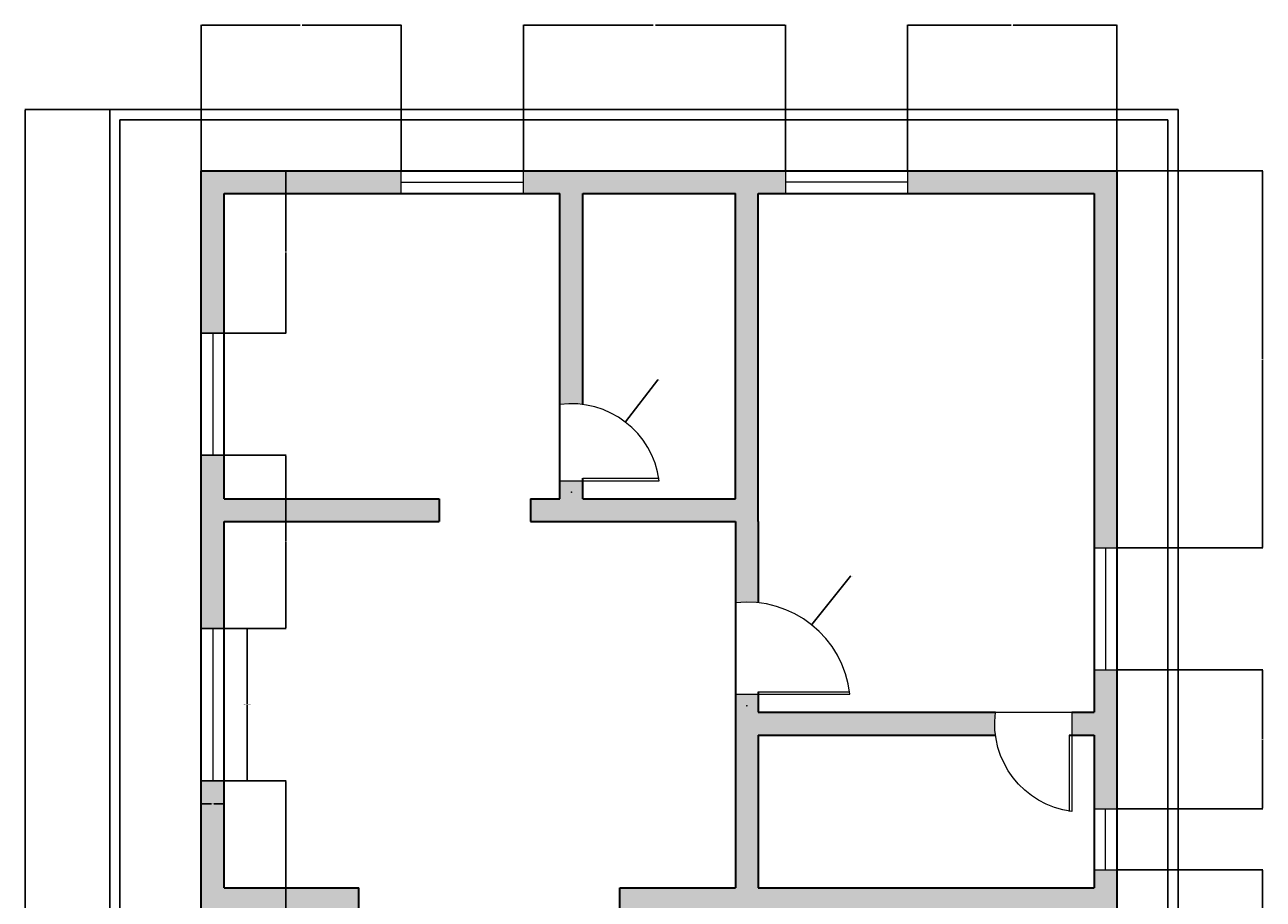
# Model space of a CAD drawing. Units: inches. Extents: x 4948 to 20975, y 6797 to 20508.
# Tile 4 of 5: x 10299 to 10786, y 20164 to 20508. Entities that reach past the tile are written whole.
import ezdxf

# ---------------------------------------------------------------- set-up
doc = ezdxf.new("R2010")
doc.units = ezdxf.units.IN
for name, color, linetype, lineweight in [('A-ANNO-DIMS', 2, 'Continuous', 18), ('A-DOOR', 3, 'Continuous', 18), ('A-GLAZ', 4, 'Continuous', 18), ('A-WALL', 7, 'Continuous', 35), ('C-PROP', 7, 'Continuous', 25)]:
    doc.layers.add(name, color=color, linetype=linetype, lineweight=lineweight)
doc.layers.add('A-WALL-PATT', color=18, linetype='Continuous', lineweight=13, true_color=0x000000)
doc.styles.get("Standard").update_dxf_attribs({"font": 'times.ttf'})
doc.dimstyles.get("Standard").update_dxf_attribs({"dimtxt": 0.18, "dimasz": 0.18, "dimexe": 0.18, "dimexo": 0.0625, "dimgap": 0.09, "dimtad": 0, "dimtih": 1, "dimtoh": 1, "dimdec": 4, "dimzin": 0, "dimdsep": 46, "dimtxsty": 'Standard', "dimcen": 0.09, "dimadec": 0, "dimazin": 0, "dimtfac": 1, "dimtdec": 4, "dimtofl": 0, "dimtmove": 0, "dimatfit": 3, "dimfxl": 1, "dimtolj": 1, "dimtzin": 0, "dimarcsym": 0})

# ---------------------------------------------------------------- blocks, each defined once
blk = doc.blocks.new('DOOR-SINGLE-36IN')
for p, q in [((9, 1), (45, 1)), ((0, 0), (9, 0)), ((9, 0), (45, 0))]:
    blk.add_line(p, q)
blk.add_arc((4.5, -4.5), 40.75, 6.3402, 96.3402)
blk = doc.blocks.new('DOOR-SINGLE-30IN')
for p, q in [((0, 0), (9, 0)), ((9, 1), (39, 1)), ((9, 0), (39, 0))]:
    blk.add_line(p, q)
blk.add_arc((4.5, -4.5), 34.79, 7.4314, 97.4314)
blk = doc.blocks.new('WIN-48IN')
for p, q in [((0, 0), (0, 9)), ((48, 0), (48, 9)), ((0, 4.5), (48, 4.5))]:
    blk.add_line(p, q)
blk = doc.blocks.new('WIN-24IN')
for p, q in [((0, 24), (9, 24)), ((4.5, 0), (4.5, 24)), ((0, 0), (9, 0))]:
    blk.add_line(p, q)
blk = doc.blocks.new('WIN-60IN')
for p, q in [((9, 60), (0, 60)), ((4.5, 60), (4.5, 0)), ((9, 0), (0, 0))]:
    blk.add_line(p, q)
blk = doc.blocks.new('*D17')
at = {"layer": 'A-ANNO-DIMS', "color": 0, "lineweight": -2, "transparency": 16777216}
for p, q in [((10377.69, 20270.68), (10386.81, 20270.68)), ((10386.63, 20270.5), (10386.63, 20240.86)), ((10386.63, 20210.86), (10386.63, 20240.5)), ((10377.69, 20210.68), (10386.81, 20210.68))]:
    blk.add_line(p, q, dxfattribs=at)
at = {"layer": 'A-ANNO-DIMS', "color": 0, "transparency": 16777216}
for points in [[(10386.6, 20270.5), (10386.66, 20270.5), (10386.63, 20270.68)], [(10386.6, 20210.86), (10386.66, 20210.86), (10386.63, 20210.68)]]:
    blk.add_solid(points, dxfattribs=at)
at = {"layer": 'Defpoints', "color": 0, "transparency": 16777216}
for p in [(10377.63, 20270.68), (10386.63, 20270.68), (10377.63, 20210.68)]:
    blk.add_point(p, dxfattribs=at)
at = {"layer": 'A-ANNO-DIMS', "color": 0, "transparency": 16777216, "insert": (10386.63, 20240.68), "char_height": 0.18, "attachment_point": 5}
blk.add_mtext('\\A1;DINING WINDOW 60 TYP.', dxfattribs=at)
blk = doc.blocks.new('*D18')
at = {"layer": 'A-ANNO-DIMS', "color": 0, "lineweight": -2, "transparency": 16777216}
for p, q in [((10368.63, 20210.62), (10368.63, 20201.5)), ((10377.63, 20210.62), (10377.63, 20201.5)), ((10368.81, 20201.68), (10372.67, 20201.68)), ((10377.45, 20201.68), (10373.59, 20201.68))]:
    blk.add_line(p, q, dxfattribs=at)
at = {"layer": 'A-ANNO-DIMS', "color": 0, "transparency": 16777216}
for points in [[(10368.81, 20201.71), (10368.81, 20201.65), (10368.63, 20201.68)], [(10377.45, 20201.71), (10377.45, 20201.65), (10377.63, 20201.68)]]:
    blk.add_solid(points, dxfattribs=at)
at = {"layer": 'Defpoints', "color": 0, "transparency": 16777216}
for p in [(10368.63, 20210.68), (10377.63, 20210.68), (10377.63, 20201.68)]:
    blk.add_point(p, dxfattribs=at)
at = {"layer": 'A-ANNO-DIMS', "color": 0, "transparency": 16777216, "insert": (10373.13, 20201.68), "char_height": 0.18, "attachment_point": 5}
blk.add_mtext('\\A1;9 TYP.', dxfattribs=at)
blk = doc.blocks.new('*D54')
at = {"layer": 'A-ANNO-DIMS', "color": 0, "lineweight": -2, "transparency": 16777216}
for p, q in [((10332.56, 20474.68), (10299.25, 20474.68)), ((10299.43, 20474.5), (10299.43, 20144.86)), ((10299.43, 19814.86), (10299.43, 20144.5)), ((10332.56, 19814.68), (10299.25, 19814.68))]:
    blk.add_line(p, q, dxfattribs=at)
at = {"layer": 'A-ANNO-DIMS', "color": 0, "transparency": 16777216}
for points in [[(10299.4, 20474.5), (10299.46, 20474.5), (10299.43, 20474.68)], [(10299.4, 19814.86), (10299.46, 19814.86), (10299.43, 19814.68)]]:
    blk.add_solid(points, dxfattribs=at)
at = {"layer": 'Defpoints', "color": 0, "transparency": 16777216}
for p in [(10299.43, 20474.68), (10332.63, 20474.68), (10332.63, 19814.68)]:
    blk.add_point(p, dxfattribs=at)
at = {"layer": 'A-ANNO-DIMS', "color": 0, "transparency": 16777216, "insert": (10299.43, 20144.68), "char_height": 0.18, "attachment_point": 5}
blk.add_mtext('\\A1;660', dxfattribs=at)
blk = doc.blocks.new('*D55')
at = {"layer": 'A-ANNO-DIMS', "color": 0, "lineweight": -2, "transparency": 16777216}
for p, q in [((10368.63, 20450.74), (10368.63, 20508.06)), ((10368.81, 20507.88), (10407.56, 20507.88)), ((10447.07, 20507.88), (10408.32, 20507.88)), ((10447.25, 20450.74), (10447.25, 20508.06))]:
    blk.add_line(p, q, dxfattribs=at)
at = {"layer": 'A-ANNO-DIMS', "color": 0, "transparency": 16777216}
for points in [[(10368.81, 20507.91), (10368.81, 20507.85), (10368.63, 20507.88)], [(10447.07, 20507.91), (10447.07, 20507.85), (10447.25, 20507.88)]]:
    blk.add_solid(points, dxfattribs=at)
at = {"layer": 'Defpoints', "color": 0, "transparency": 16777216}
for p in [(10447.25, 20507.88), (10368.63, 20450.68), (10447.25, 20450.68)]:
    blk.add_point(p, dxfattribs=at)
at = {"layer": 'A-ANNO-DIMS', "color": 0, "transparency": 16777216, "insert": (10407.94, 20507.88), "char_height": 0.18, "attachment_point": 5}
blk.add_mtext('\\A1;78.62', dxfattribs=at)
blk = doc.blocks.new('*D56')
at = {"layer": 'A-ANNO-DIMS', "color": 0, "lineweight": -2, "transparency": 16777216}
for p, q in [((10495.25, 20450.74), (10495.25, 20508.06)), ((10495.43, 20507.88), (10546.33, 20507.88)), ((10598.11, 20507.88), (10547.2, 20507.88)), ((10598.29, 20450.74), (10598.29, 20508.06))]:
    blk.add_line(p, q, dxfattribs=at)
at = {"layer": 'A-ANNO-DIMS', "color": 0, "transparency": 16777216}
for points in [[(10495.43, 20507.91), (10495.43, 20507.85), (10495.25, 20507.88)], [(10598.11, 20507.91), (10598.11, 20507.85), (10598.29, 20507.88)]]:
    blk.add_solid(points, dxfattribs=at)
at = {"layer": 'Defpoints', "color": 0, "transparency": 16777216}
for p in [(10598.29, 20507.88), (10495.25, 20450.68), (10598.29, 20450.68)]:
    blk.add_point(p, dxfattribs=at)
at = {"layer": 'A-ANNO-DIMS', "color": 0, "transparency": 16777216, "insert": (10546.77, 20507.88), "char_height": 0.18, "attachment_point": 5}
blk.add_mtext('\\A1;103.04', dxfattribs=at)
blk = doc.blocks.new('*D57')
at = {"layer": 'A-ANNO-DIMS', "color": 0, "lineweight": -2, "transparency": 16777216}
for p, q in [((10646.29, 20450.74), (10646.29, 20508.06)), ((10646.47, 20507.88), (10687.08, 20507.88)), ((10728.45, 20507.88), (10687.83, 20507.88)), ((10728.63, 20450.74), (10728.63, 20508.06))]:
    blk.add_line(p, q, dxfattribs=at)
at = {"layer": 'A-ANNO-DIMS', "color": 0, "transparency": 16777216}
for points in [[(10646.47, 20507.91), (10646.47, 20507.85), (10646.29, 20507.88)], [(10728.45, 20507.91), (10728.45, 20507.85), (10728.63, 20507.88)]]:
    blk.add_solid(points, dxfattribs=at)
at = {"layer": 'Defpoints', "color": 0, "transparency": 16777216}
for p in [(10728.63, 20507.88), (10646.29, 20450.68), (10728.63, 20450.68)]:
    blk.add_point(p, dxfattribs=at)
at = {"layer": 'A-ANNO-DIMS', "color": 0, "transparency": 16777216, "insert": (10687.46, 20507.88), "char_height": 0.18, "attachment_point": 5}
blk.add_mtext('\\A1;82.34', dxfattribs=at)
blk = doc.blocks.new('*D60')
at = {"layer": 'A-ANNO-DIMS', "color": 0, "lineweight": -2, "transparency": 16777216}
for p, q in [((10368.69, 20450.68), (10402.01, 20450.68)), ((10401.83, 20450.5), (10401.83, 20418.91)), ((10401.83, 20386.95), (10401.83, 20418.54)), ((10368.69, 20386.77), (10402.01, 20386.77))]:
    blk.add_line(p, q, dxfattribs=at)
at = {"layer": 'A-ANNO-DIMS', "color": 0, "transparency": 16777216}
for points in [[(10401.8, 20450.5), (10401.86, 20450.5), (10401.83, 20450.68)], [(10401.8, 20386.95), (10401.86, 20386.95), (10401.83, 20386.77)]]:
    blk.add_solid(points, dxfattribs=at)
at = {"layer": 'Defpoints', "color": 0, "transparency": 16777216}
for p in [(10368.63, 20450.68), (10368.63, 20386.77), (10401.83, 20386.77)]:
    blk.add_point(p, dxfattribs=at)
at = {"layer": 'A-ANNO-DIMS', "color": 0, "transparency": 16777216, "insert": (10401.83, 20418.73), "char_height": 0.18, "attachment_point": 5}
blk.add_mtext('\\A1;63.91', dxfattribs=at)
blk = doc.blocks.new('*D61')
at = {"layer": 'A-ANNO-DIMS', "color": 0, "lineweight": -2, "transparency": 16777216}
for p, q in [((10368.69, 20338.77), (10402.01, 20338.77)), ((10401.83, 20338.59), (10401.83, 20304.91)), ((10401.83, 20270.86), (10401.83, 20304.54)), ((10368.69, 20270.68), (10402.01, 20270.68))]:
    blk.add_line(p, q, dxfattribs=at)
at = {"layer": 'A-ANNO-DIMS', "color": 0, "transparency": 16777216}
for points in [[(10401.8, 20338.59), (10401.86, 20338.59), (10401.83, 20338.77)], [(10401.8, 20270.86), (10401.86, 20270.86), (10401.83, 20270.68)]]:
    blk.add_solid(points, dxfattribs=at)
at = {"layer": 'Defpoints', "color": 0, "transparency": 16777216}
for p in [(10368.63, 20338.77), (10368.63, 20270.68), (10401.83, 20270.68)]:
    blk.add_point(p, dxfattribs=at)
at = {"layer": 'A-ANNO-DIMS', "color": 0, "transparency": 16777216, "insert": (10401.83, 20304.73), "char_height": 0.18, "attachment_point": 5}
blk.add_mtext('\\A1;68.09', dxfattribs=at)
blk = doc.blocks.new('*D62')
at = {"layer": 'A-ANNO-DIMS', "color": 0, "lineweight": -2, "transparency": 16777216}
for p, q in [((10368.69, 20210.68), (10402.01, 20210.68)), ((10401.83, 20210.5), (10401.83, 20147.11)), ((10401.83, 20083.36), (10401.83, 20146.75)), ((10368.69, 20083.18), (10402.01, 20083.18))]:
    blk.add_line(p, q, dxfattribs=at)
at = {"layer": 'A-ANNO-DIMS', "color": 0, "transparency": 16777216}
for points in [[(10401.8, 20210.5), (10401.86, 20210.5), (10401.83, 20210.68)], [(10401.8, 20083.36), (10401.86, 20083.36), (10401.83, 20083.18)]]:
    blk.add_solid(points, dxfattribs=at)
at = {"layer": 'Defpoints', "color": 0, "transparency": 16777216}
for p in [(10368.63, 20210.68), (10368.63, 20083.18), (10401.83, 20083.18)]:
    blk.add_point(p, dxfattribs=at)
at = {"layer": 'A-ANNO-DIMS', "color": 0, "transparency": 16777216, "insert": (10401.83, 20146.93), "char_height": 0.18, "attachment_point": 5}
blk.add_mtext('\\A1;127.5', dxfattribs=at)
blk = doc.blocks.new('*D66')
at = {"layer": 'A-ANNO-DIMS', "color": 0, "lineweight": -2, "transparency": 16777216}
for p, q in [((10728.69, 20175.78), (10786.01, 20175.78)), ((10785.83, 20175.6), (10785.83, 20137.64)), ((10785.83, 20099.31), (10785.83, 20137.27)), ((10728.69, 20099.13), (10786.01, 20099.13))]:
    blk.add_line(p, q, dxfattribs=at)
at = {"layer": 'A-ANNO-DIMS', "color": 0, "transparency": 16777216}
for points in [[(10785.8, 20175.6), (10785.86, 20175.6), (10785.83, 20175.78)], [(10785.8, 20099.31), (10785.86, 20099.31), (10785.83, 20099.13)]]:
    blk.add_solid(points, dxfattribs=at)
at = {"layer": 'Defpoints', "color": 0, "transparency": 16777216}
for p in [(10728.63, 20175.78), (10785.83, 20175.78), (10728.63, 20099.13)]:
    blk.add_point(p, dxfattribs=at)
at = {"layer": 'A-ANNO-DIMS', "color": 0, "transparency": 16777216, "insert": (10785.83, 20137.46), "char_height": 0.18, "attachment_point": 5}
blk.add_mtext('\\A1;76.65', dxfattribs=at)
blk = doc.blocks.new('*D67')
at = {"layer": 'A-ANNO-DIMS', "color": 0, "lineweight": -2, "transparency": 16777216}
for p, q in [((10728.69, 20254.38), (10786.01, 20254.38)), ((10785.83, 20254.2), (10785.83, 20227.26)), ((10785.83, 20199.96), (10785.83, 20226.9)), ((10728.69, 20199.78), (10786.01, 20199.78))]:
    blk.add_line(p, q, dxfattribs=at)
at = {"layer": 'A-ANNO-DIMS', "color": 0, "transparency": 16777216}
for points in [[(10785.8, 20254.2), (10785.86, 20254.2), (10785.83, 20254.38)], [(10785.8, 20199.96), (10785.86, 20199.96), (10785.83, 20199.78)]]:
    blk.add_solid(points, dxfattribs=at)
at = {"layer": 'Defpoints', "color": 0, "transparency": 16777216}
for p in [(10728.63, 20254.38), (10785.83, 20254.38), (10728.63, 20199.78)]:
    blk.add_point(p, dxfattribs=at)
at = {"layer": 'A-ANNO-DIMS', "color": 0, "transparency": 16777216, "insert": (10785.83, 20227.08), "char_height": 0.18, "attachment_point": 5}
blk.add_mtext('\\A1;54.61', dxfattribs=at)
blk = doc.blocks.new('*D68')
at = {"layer": 'A-ANNO-DIMS', "color": 0, "lineweight": -2, "transparency": 16777216}
for p, q in [((10728.69, 20450.68), (10786.01, 20450.68)), ((10785.83, 20450.5), (10785.83, 20376.71)), ((10785.83, 20302.56), (10785.83, 20376.35)), ((10728.69, 20302.38), (10786.01, 20302.38))]:
    blk.add_line(p, q, dxfattribs=at)
at = {"layer": 'A-ANNO-DIMS', "color": 0, "transparency": 16777216}
for points in [[(10785.8, 20450.5), (10785.86, 20450.5), (10785.83, 20450.68)], [(10785.8, 20302.56), (10785.86, 20302.56), (10785.83, 20302.38)]]:
    blk.add_solid(points, dxfattribs=at)
at = {"layer": 'Defpoints', "color": 0, "transparency": 16777216}
for p in [(10728.63, 20450.68), (10785.83, 20450.68), (10728.63, 20302.38)]:
    blk.add_point(p, dxfattribs=at)
at = {"layer": 'A-ANNO-DIMS', "color": 0, "transparency": 16777216, "insert": (10785.83, 20376.53), "char_height": 0.18, "attachment_point": 5}
blk.add_mtext('\\A1;148.3', dxfattribs=at)
blk = doc.blocks.new('*D93')
at = {"layer": 'A-ANNO-DIMS', "color": 0, "lineweight": -2, "transparency": 16777216}
for p, q in [((10623.86, 20291.2), (10608.7, 20272.25)), ((10624.04, 20291.2), (10623.86, 20291.2)), ((10583.04, 20240.29), (10583.22, 20240.29)), ((10583.13, 20240.2), (10583.13, 20240.38))]:
    blk.add_line(p, q, dxfattribs=at)
at = {"layer": 'A-ANNO-DIMS', "color": 0, "transparency": 16777216}
blk.add_solid([(10608.67, 20272.27), (10608.72, 20272.23), (10608.58, 20272.11)], dxfattribs=at)
at = {"layer": 'Defpoints', "color": 0, "transparency": 16777216}
for p in [(10608.58, 20272.11), (10583.13, 20240.29)]:
    blk.add_point(p, dxfattribs=at)
at = {"layer": 'A-ANNO-DIMS', "color": 0, "transparency": 16777216, "insert": (10624.7, 20291.2), "char_height": 0.18, "attachment_point": 5}
blk.add_mtext('\\A1;2X R40.75', dxfattribs=at)
blk = doc.blocks.new('*D94')
at = {"layer": 'A-ANNO-DIMS', "color": 0, "lineweight": -2, "transparency": 16777216}
for p, q in [((10548.07, 20368.37), (10535.45, 20351.97)), ((10548.25, 20368.37), (10548.07, 20368.37)), ((10514.04, 20324.25), (10514.22, 20324.25)), ((10514.13, 20324.16), (10514.13, 20324.34))]:
    blk.add_line(p, q, dxfattribs=at)
at = {"layer": 'A-ANNO-DIMS', "color": 0, "transparency": 16777216}
blk.add_solid([(10535.43, 20351.98), (10535.47, 20351.95), (10535.34, 20351.82)], dxfattribs=at)
at = {"layer": 'Defpoints', "color": 0, "transparency": 16777216}
for p in [(10535.34, 20351.82), (10514.13, 20324.25)]:
    blk.add_point(p, dxfattribs=at)
at = {"layer": 'A-ANNO-DIMS', "color": 0, "transparency": 16777216, "insert": (10548.72, 20368.37), "char_height": 0.18, "attachment_point": 5}
blk.add_mtext('\\A1;R34.79', dxfattribs=at)

msp = doc.modelspace()

# ---------------------------------------------------------------- hatches: boundary and pattern name
at = {"layer": 'A-WALL-PATT'}
h = msp.add_hatch(color=256, dxfattribs=at)
h.dxf.hatch_style = 1
h.paths.add_polyline_path([(10447.2486, 20450.6802), (10368.6272, 20450.6802), (10368.6272, 20386.7714), (10377.6272, 20386.7714), (10377.6272, 20441.6802), (10447.2486, 20441.6802)])
h.paths.add_polyline_path([(10598.2871, 20450.6802), (10495.2486, 20450.6802), (10495.2486, 20441.6802), (10509.6272, 20441.6802), (10509.6272, 20358.7457, -0.06494234), (10518.6272, 20358.7457), (10518.6272, 20441.6802), (10578.6272, 20441.6802), (10578.6272, 20321.6802), (10518.6272, 20321.6802), (10518.6272, 20328.7457), (10509.6272, 20328.7457), (10509.6272, 20321.6802), (10498.0955, 20321.6802), (10498.0955, 20312.6802), (10578.6272, 20312.6802), (10578.6272, 20280.7888, -0.05538514), (10587.6272, 20280.7888), (10587.6272, 20312.6802), (10587.6272, 20441.6802), (10598.2871, 20441.6802)])
h.paths.add_polyline_path([(10728.6272, 20450.6802), (10646.2871, 20450.6802), (10646.2871, 20441.6802), (10719.6272, 20441.6802), (10719.6272, 20302.385), (10728.6272, 20302.385)])
h.paths.add_polyline_path([(10377.6272, 20312.6802), (10462.0955, 20312.6802), (10462.0955, 20321.6802), (10377.6272, 20321.6802), (10377.6272, 20338.7714), (10368.6272, 20338.7714), (10368.6272, 20270.6802), (10377.6272, 20270.6802)])
h.paths.add_polyline_path([(10728.6272, 20175.7784), (10719.6272, 20175.7784), (10719.6272, 20168.6802), (10587.6272, 20168.6802), (10587.6272, 20228.6802), (10680.8649, 20228.6802, -0.06494234), (10680.8649, 20237.6802), (10587.6272, 20237.6802), (10587.6272, 20244.7888), (10578.6272, 20244.7888), (10578.6272, 20228.6802), (10578.6272, 20168.6802), (10533.2309, 20168.6802), (10533.2309, 20159.6802), (10578.6272, 20159.6802), (10578.6272, 20069.7581, -0.05538514), (10587.6272, 20069.7581), (10587.6272, 20159.6802), (10719.6272, 20159.6802), (10719.6272, 20099.1317), (10728.6272, 20099.1317)])
h.paths.add_polyline_path([(10728.6272, 20254.385), (10719.6272, 20254.385), (10719.6272, 20237.6802), (10710.8649, 20237.6802), (10710.8649, 20228.6802), (10719.6272, 20228.6802), (10719.6272, 20199.7784), (10728.6272, 20199.7784)])
h.paths.add_polyline_path([(10728.6272, 20051.1317), (10719.6272, 20051.1317), (10719.6272, 20027.6802), (10712.464, 20027.6802), (10712.464, 20018.6802), (10719.6272, 20018.6802), (10719.6272, 20000.6802), (10728.6272, 20000.6802)])
h.paths.add_polyline_path([(10728.6272, 19976.6802), (10719.6272, 19976.6802), (10719.6272, 19958.6802), (10587.6272, 19958.6802), (10587.6272, 20018.6802), (10682.464, 20018.6802, -0.06494234), (10682.464, 20027.6802), (10587.6272, 20027.6802), (10587.6272, 20033.7581), (10578.6272, 20033.7581), (10578.6272, 19958.6802), (10496.0899, 19958.6802), (10496.0899, 19949.6802), (10578.6272, 19949.6802), (10587.6272, 19949.6802), (10719.6272, 19949.6802), (10719.6272, 19874.6802), (10578.6272, 19874.6802), (10578.6272, 19865.6802), (10728.6272, 19865.6802)])
h.paths.add_polyline_path([(10412.0899, 19958.6802), (10377.6272, 19958.6802), (10377.6272, 20035.1802), (10368.6272, 20035.1802), (10368.6272, 19949.6802), (10377.6272, 19949.6802), (10412.0899, 19949.6802)])
h.paths.add_polyline_path([(10377.6272, 20159.6802), (10430.5935, 20159.6802), (10430.5935, 20168.6802), (10377.6272, 20168.6802), (10377.6272, 20210.6802), (10368.6272, 20210.6802), (10368.6272, 20083.1802), (10377.6272, 20083.1802)])

# ---------------------------------------------------------------- linework, layer by layer
at = {"layer": 'A-DOOR'}
msp.add_line((10680.8649, 20237.6802), (10710.8649, 20237.6802), dxfattribs=at)
at = {"layer": 'A-WALL'}
for p, q in [((10368.6272, 20450.6802), (10728.6272, 20450.6802)), ((10368.6272, 19949.6802), (10368.6272, 20450.6802)), ((10728.6272, 20450.6802), (10728.6272, 19865.6802)), ((10377.6272, 20441.6802), (10509.6272, 20441.6802)), ((10377.6272, 20321.6802), (10377.6272, 20441.6802)), ((10509.6272, 20321.6802), (10509.6272, 20441.6802)), ((10518.6272, 20441.6802), (10578.6272, 20441.6802)), ((10518.6272, 20358.7457), (10518.6272, 20441.6802)), ((10578.6272, 20321.6802), (10578.6272, 20441.6802)), ((10587.6272, 20441.6802), (10719.6272, 20441.6802)), ((10587.6272, 20312.6802), (10587.6272, 20441.6802)), ((10719.6272, 20441.6802), (10719.6272, 20237.6802)), ((10518.6272, 20321.6802), (10518.6272, 20329.7457)), ((10377.6272, 20321.6802), (10462.0955, 20321.6802)), ((10462.0955, 20321.6802), (10462.0955, 20312.6802)), ((10498.0955, 20321.6802), (10509.6272, 20321.6802)), ((10498.0955, 20321.6802), (10498.0955, 20312.6802)), ((10518.6272, 20321.6802), (10578.6272, 20321.6802)), ((10377.6272, 20312.6802), (10462.0955, 20312.6802)), ((10377.6272, 20168.6802), (10377.6272, 20312.6802)), ((10498.0955, 20312.6802), (10578.6272, 20312.6802)), ((10578.6272, 20312.6802), (10578.6272, 20228.6802)), ((10587.6272, 20312.6802), (10587.6272, 20280.7888)), ((10587.6272, 20245.7888), (10587.6272, 20237.6802)), ((10587.6272, 20237.6802), (10680.8649, 20237.6802)), ((10710.8649, 20237.6802), (10719.6272, 20237.6802)), ((10578.6272, 20228.6802), (10578.6272, 20168.6802)), ((10587.6272, 20228.6802), (10680.8649, 20228.6802)), ((10587.6272, 20228.6802), (10587.6272, 20168.6802)), ((10709.8649, 20228.6802), (10719.6272, 20228.6802)), ((10719.6272, 20228.6802), (10719.6272, 20168.6802)), ((10377.6272, 20168.6802), (10430.5935, 20168.6802)), ((10430.5935, 20159.6802), (10430.5935, 20168.6802)), ((10533.2309, 20168.6802), (10578.6272, 20168.6802)), ((10533.2309, 20159.6802), (10533.2309, 20168.6802)), ((10587.6272, 20168.6802), (10719.6272, 20168.6802))]:
    msp.add_line(p, q, dxfattribs=at)
at = {"layer": 'C-PROP'}
for p, q in [((10332.6272, 20474.6802), (10752.6272, 20474.6802)), ((10332.6272, 19814.6802), (10332.6272, 20474.6802)), ((10752.6272, 20474.6802), (10752.6272, 19814.6802)), ((10336.6272, 20470.6802), (10748.6272, 20470.6802)), ((10336.6272, 19818.6802), (10336.6272, 20470.6802)), ((10748.6272, 20470.6802), (10748.6272, 19818.6802))]:
    msp.add_line(p, q, dxfattribs=at)

# ---------------------------------------------------------------- block references
at = {"layer": 'A-DOOR'}
for name, p in [('DOOR-SINGLE-30IN', (10509.6273, 20328.7452)), ('DOOR-SINGLE-36IN', (10578.6273, 20244.7892))]:
    msp.add_blockref(name, p, dxfattribs=at)
at = {"layer": 'A-DOOR', "extrusion": (0, 0, -1), "zscale": -1, "rotation": 270.000000000009}
msp.add_blockref('DOOR-SINGLE-30IN', (-10710.8653, 20237.6802), dxfattribs=at)
at = {"layer": 'A-GLAZ'}
for name, p in [('WIN-48IN', (10447.2483, 20441.6802)), ('WIN-60IN', (10368.6273, 20210.6802)), ('WIN-24IN', (10719.6273, 20175.7782))]:
    msp.add_blockref(name, p, dxfattribs=at)
for p, rotation in [((10646.2875, 20450.6803), 180), ((10368.6272, 20386.7717), 269.9999999999955), ((10719.6272, 20302.3853), 269.9999999999998)]:
    msp.add_blockref('WIN-48IN', p, dxfattribs=dict(at, rotation=rotation))

# ---------------------------------------------------------------- dimensions: what is measured, and where the dimension line sits
at = {"layer": 'A-ANNO-DIMS'}
for base, p1, p2, picture, middle in [((10447.2486, 20507.8802), (10368.6272, 20450.6802), (10447.2486, 20450.6802), '*D55', (10407.9379, 20507.8802)), ((10598.2871, 20507.8802), (10495.2486, 20450.6802), (10598.2871, 20450.6802), '*D56', (10546.7679, 20507.8802)), ((10728.6272, 20507.8802), (10646.2871, 20450.6802), (10728.6272, 20450.6802), '*D57', (10687.4572, 20507.8802))]:
    dim = msp.add_linear_dim(base=base, p1=p1, p2=p2, dimstyle='Standard', override={"dimdec": 2, "dimlfac": 1, "dimrnd": 0, "dimzin": 0, "dimdsep": 46, "dimlunit": 2}, dxfattribs=at)
    dim.commit()
    dim.dimension.update_dxf_attribs({"geometry": picture, "text_midpoint": middle})
for base, p1, p2, angle, override, picture, middle in [((10299.4272, 20474.6802), (10332.6272, 19814.6802), (10332.6272, 20474.6802), 90, {"dimdec": 0, "dimlfac": 1, "dimrnd": 0, "dimzin": 0, "dimdsep": 46, "dimlunit": 2}, '*D54', (10299.4272, 20144.6802)), ((10401.8272, 20386.7714), (10368.6272, 20450.6802), (10368.6272, 20386.7714), 270, {"dimdec": 2, "dimlfac": 1, "dimrnd": 0, "dimzin": 0, "dimdsep": 46, "dimlunit": 2}, '*D60', (10401.8272, 20418.7258)), ((10785.8272, 20450.6802), (10728.6272, 20302.385), (10728.6272, 20450.6802), 90, {"dimdec": 1, "dimlfac": 1, "dimrnd": 0, "dimzin": 0, "dimdsep": 46, "dimlunit": 2}, '*D68', (10785.8272, 20376.5326)), ((10401.8272, 20270.6802), (10368.6272, 20338.7714), (10368.6272, 20270.6802), 270, {"dimdec": 2, "dimlfac": 1, "dimrnd": 0, "dimzin": 0, "dimdsep": 46, "dimlunit": 2}, '*D61', (10401.8272, 20304.7258)), ((10785.8272, 20254.385), (10728.6272, 20199.7784), (10728.6272, 20254.385), 90, {"dimdec": 2, "dimlfac": 1, "dimrnd": 0, "dimzin": 0, "dimdsep": 46, "dimlunit": 2}, '*D67', (10785.8272, 20227.0817)), ((10401.8272, 20083.1802), (10368.6272, 20210.6802), (10368.6272, 20083.1802), 270, {"dimdec": 1, "dimlfac": 1, "dimrnd": 0, "dimzin": 0, "dimdsep": 46, "dimlunit": 2}, '*D62', (10401.8272, 20146.9302)), ((10785.8272, 20175.7784), (10728.6272, 20099.1317), (10728.6272, 20175.7784), 90, {"dimdec": 2, "dimlfac": 1, "dimrnd": 0, "dimzin": 0, "dimdsep": 46, "dimlunit": 2}, '*D66', (10785.8272, 20137.4551))]:
    dim = msp.add_linear_dim(base=base, p1=p1, p2=p2, angle=angle, dimstyle='Standard', override=override, dxfattribs=at)
    dim.commit()
    dim.dimension.update_dxf_attribs({"geometry": picture, "text_midpoint": middle})
dim = msp.add_radius_dim(center=(10514.1272, 20324.2457), mpoint=(10535.3401, 20351.8231), dimstyle='Standard', override={"dimdec": 2, "dimlfac": 1, "dimrnd": 0, "dimzin": 0, "dimdsep": 46, "dimlunit": 2}, dxfattribs=at)
dim.commit()
dim.dimension.update_dxf_attribs({"geometry": '*D94', "text_midpoint": (10548.7174, 20368.3695), "dimtype": 164})
dim = msp.add_radius_dim(center=(10583.1272, 20240.2888), mpoint=(10608.5828, 20272.1088), text='2X <>', dimstyle='Standard', override={"dimdec": 2, "dimlfac": 1, "dimrnd": 0, "dimzin": 0, "dimdsep": 46, "dimlunit": 2}, dxfattribs=at)
dim.commit()
dim.dimension.update_dxf_attribs({"geometry": '*D93', "text_midpoint": (10624.6979, 20291.2008), "dimtype": 164})
dim = msp.add_linear_dim(base=(10386.6272, 20270.6802), p1=(10377.6272, 20210.6802), p2=(10377.6272, 20270.6802), angle=90, text='DINING WINDOW <> TYP.', dimstyle='Standard', override={"dimdec": 0, "dimlfac": 1, "dimrnd": 0, "dimzin": 0, "dimdsep": 46, "dimlunit": 2}, dxfattribs=at)
dim.commit()
dim.dimension.update_dxf_attribs({"geometry": '*D17', "text_midpoint": (10386.6272, 20240.6802)})
dim = msp.add_linear_dim(base=(10377.6272, 20201.6802), p1=(10368.6272, 20210.6802), p2=(10377.6272, 20210.6802), text='<> TYP.', dimstyle='Standard', override={"dimdec": 0, "dimlfac": 1, "dimrnd": 0, "dimzin": 0, "dimdsep": 46, "dimlunit": 2}, dxfattribs=at)
dim.commit()
dim.dimension.update_dxf_attribs({"geometry": '*D18', "text_midpoint": (10373.1272, 20201.6802)})

doc.saveas('drawing.dxf')
